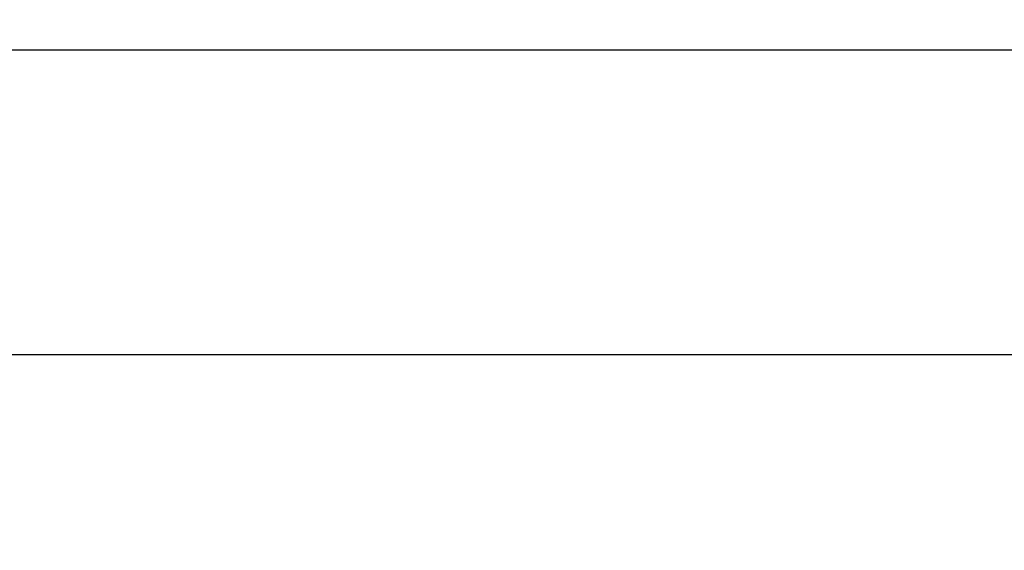
# Model space of a CAD drawing. Units: inches. Extents: x 3283068 to 3284536, y 3240756 to 3241803.
# Tile 13 of 19: x 3283383 to 3283598, y 3241688 to 3241803. Entities that reach past the tile are written whole.
import ezdxf

# ---------------------------------------------------------------- set-up
doc = ezdxf.new("R2010")
doc.units = ezdxf.units.IN
doc.layers.add('A-ANNO-DIMS', color=2, linetype='Continuous', lineweight=18)
doc.layers.add('C-PROP', color=7, linetype='Continuous', lineweight=25)
doc.styles.get("Standard").update_dxf_attribs({"font": 'arial.ttf'})
doc.dimstyles.new('ISO-25', dxfattribs={"dimtxt": 5, "dimasz": 2.5, "dimexe": 1.25, "dimexo": 0.625, "dimtad": 1, "dimlunit": 4, "dimtxsty": 'Standard', "dimblk": 'ARCHTICK', "dimcen": 2.5, "dimadec": 0, "dimazin": 0, "dimtfac": 1, "dimtmove": 0, "dimatfit": 3, "dimfxl": 1, "dimarcsym": 0})

# ---------------------------------------------------------------- blocks, each defined once
blk = doc.blocks.new('_ArchTick')
at = {"color": 0, "linetype": 'ByBlock', "const_width": 0.15}
blk.add_lwpolyline([(-0.5, -0.5), (0.5, 0.5)], dxfattribs=at)
blk = doc.blocks.new('*D63')
at = {"layer": 'A-ANNO-DIMS', "color": 0, "lineweight": -2, "transparency": 16777216}
for p, q in [((3283248.09, 3241083.23), (3283248.09, 3241798.08)), ((3284328.09, 3241083.23), (3284328.09, 3241798.08)), ((3283248.09, 3241796.83), (3284328.09, 3241796.83))]:
    blk.add_line(p, q, dxfattribs=at)
at = {"layer": 'Defpoints', "color": 0, "transparency": 16777216}
for p in [(3284328.09, 3241796.83), (3283248.09, 3241082.6), (3284328.09, 3241082.6)]:
    blk.add_point(p, dxfattribs=at)
at = {"layer": 'A-ANNO-DIMS', "color": 0, "lineweight": -2, "transparency": 16777216, "xscale": 2.5, "yscale": 2.5, "zscale": 2.5, "rotation": 180}
blk.add_blockref('_ArchTick', (3283248.09, 3241796.83), dxfattribs=at)
at = {"layer": 'A-ANNO-DIMS', "color": 0, "lineweight": -2, "transparency": 16777216, "xscale": 2.5, "yscale": 2.5, "zscale": 2.5}
blk.add_blockref('_ArchTick', (3284328.09, 3241796.83), dxfattribs=at)
at = {"layer": 'A-ANNO-DIMS', "color": 0, "transparency": 16777216, "insert": (3283788.09, 3241800.01), "char_height": 5, "attachment_point": 5}
blk.add_mtext('90\'-0"', dxfattribs=at)

msp = doc.modelspace()

# ---------------------------------------------------------------- linework, layer by layer
at = {"layer": 'C-PROP'}
msp.add_line((3283248.089, 3241730.602), (3284328.089, 3241730.602), dxfattribs=at)

# ---------------------------------------------------------------- dimensions: what is measured, and where the dimension line sits
at = {"layer": 'A-ANNO-DIMS'}
dim = msp.add_linear_dim(base=(3284328.089, 3241796.827), p1=(3283248.089, 3241082.602), p2=(3284328.089, 3241082.602), dimstyle='ISO-25', override={"dimdec": 1, "dimlfac": 1, "dimrnd": 0, "dimzin": 1, "dimdsep": 46, "dimlunit": 4, "dimfrac": 2}, dxfattribs=at)
dim.commit()
dim.dimension.update_dxf_attribs({"geometry": '*D63', "text_midpoint": (3283788.089, 3241800.005)})

doc.saveas('drawing.dxf')
